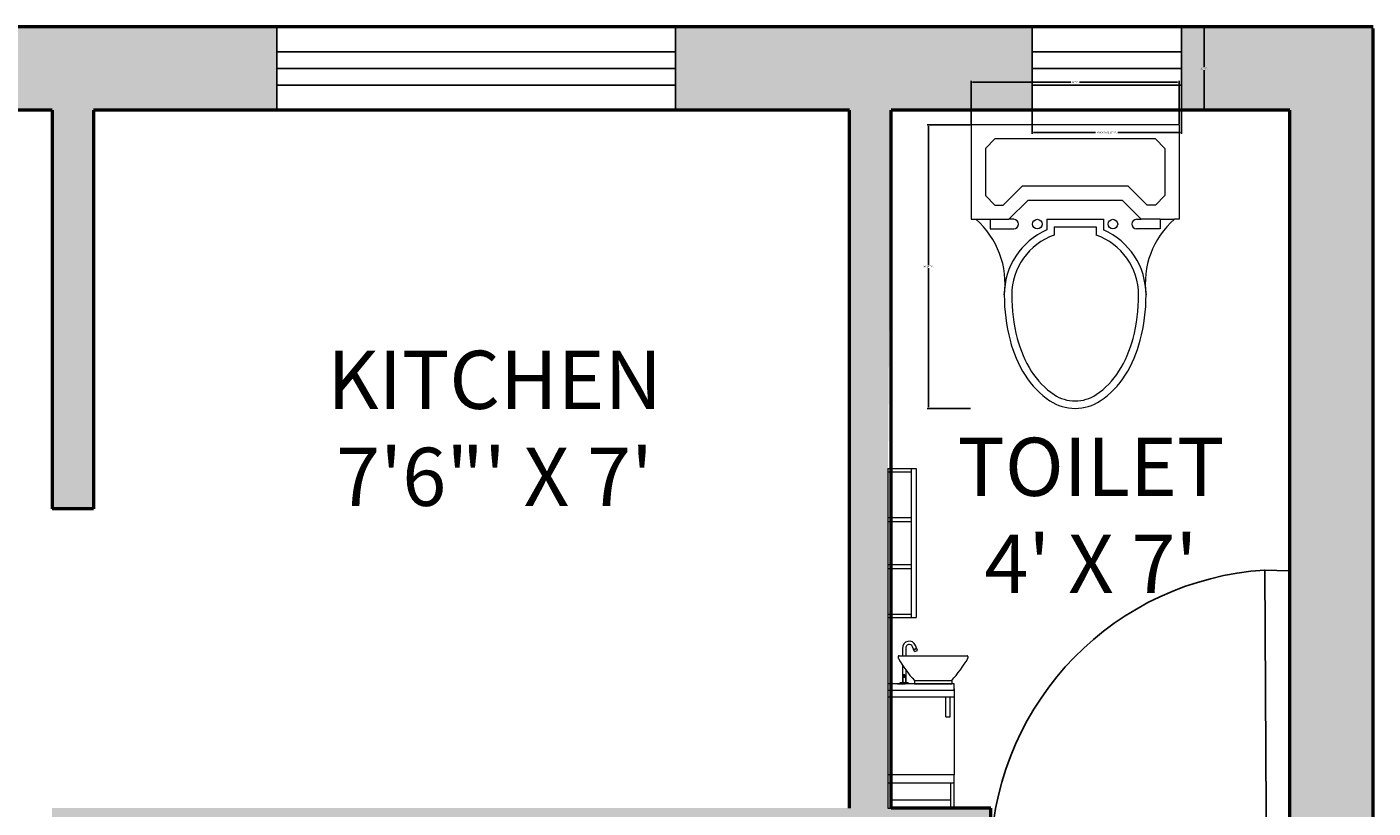
# Model space of a CAD drawing. Units: inches. Extents: x 1771 to 3025, y 319 to 889.
# Tile 12 of 35: x 1939 to 2101, y 795 to 889. Entities that reach past the tile are written whole.
import ezdxf

# ---------------------------------------------------------------- set-up
doc = ezdxf.new("R2010")
doc.units = ezdxf.units.IN
doc.header["$MEASUREMENT"] = 0
for name, color, linetype, lineweight in [('A-ANNO-DIMS', 2, 'Continuous', 18), ('A-AREA-IDEN', 241, 'Continuous', 25), ('A-DOOR', 4, 'Continuous', 25), ('A-FLOR-FIXT', 8, 'Continuous', 18), ('A-GLAZ', 40, 'Continuous', 25), ('A-WALL', 7, 'Continuous', 50), ('A-WALL-PATT', 254, 'Continuous', 13)]:
    doc.layers.add(name, color=color, linetype=linetype, lineweight=lineweight)
doc.styles.get("Standard").update_dxf_attribs({"font": 'arial.ttf'})
doc.dimstyles.get("Standard").update_dxf_attribs({"dimtxt": 0.18, "dimasz": 0.18, "dimexe": 0.18, "dimexo": 0.0625, "dimgap": 0.09, "dimtad": 0, "dimtih": 1, "dimtoh": 1, "dimdec": 4, "dimzin": 0, "dimdsep": 46, "dimtxsty": 'Standard', "dimcen": 0.09, "dimadec": 0, "dimazin": 0, "dimtfac": 1, "dimtdec": 4, "dimtofl": 0, "dimtmove": 0, "dimatfit": 3, "dimfxl": 1, "dimtolj": 1, "dimtzin": 0, "dimarcsym": 0})

# ---------------------------------------------------------------- blocks, each defined once
blk = doc.blocks.new('A$C098B081F')
for p, q in [((558.8, 762), (0, 762)), ((0, 762), (0, 508)), ((558.8, 762), (558.8, 508)), ((63.5, 723.9), (38.1, 698.5)), ((495.3, 723.9), (63.5, 723.9)), ((520.7, 698.5), (495.3, 723.9)), ((38.1, 698.5), (38.1, 571.5)), ((520.7, 698.5), (520.7, 571.5)), ((136.6, 596.9), (85.8, 546.1)), ((422.2, 596.9), (136.6, 596.9)), ((422.2, 596.9), (473, 546.1)), ((38.1, 571.5), (63.5, 546.1)), ((63.5, 546.1), (85.8, 546.1)), ((152.4, 558.8), (101.6, 508)), ((406.4, 558.8), (152.4, 558.8)), ((406.4, 558.8), (457.2, 508)), ((495.3, 546.1), (473, 546.1)), ((495.3, 546.1), (520.7, 571.5)), ((0, 508), (12.7, 508)), ((12.7, 508), (101.6, 508)), ((50.8, 508), (50.8, 482.6)), ((50.8, 508), (101.6, 508)), ((114.3, 508), (101.6, 508)), ((203.2, 508), (203.2, 479.4)), ((203.2, 508), (355.6, 508)), ((355.6, 508), (355.6, 479.4)), ((444.5, 508), (457.2, 508)), ((508, 508), (457.2, 508)), ((508, 508), (546.1, 508)), ((508, 508), (508, 482.6)), ((558.8, 508), (546.1, 508)), ((50.8, 482.6), (114.3, 482.6)), ((223.2, 488), (223.2, 465.8)), ((223.2, 488), (335.6, 488)), ((335.6, 488), (335.6, 465.8)), ((508, 482.6), (444.5, 482.6))]:
    blk.add_line(p, q)
for centre in [(177.8, 495.3), (381, 495.3)]:
    blk.add_circle(centre, 12.7)
for centre, radius, start, end in [((-137.5, 335.8), 228.5, 352.2011, 48.911), ((114.3, 495.3), 12.7, 270, 90), ((444.5, 495.3), 12.7, 90, 270), ((696.3, 335.8), 228.5, 131.089, 187.7989), ((279.4, 304.8), 190.5, 113.5782, 180), ((279.4, 304.8), 190.5, 0, 66.4218), ((279.4, 304.8), 170.5, 109.2456, 180), ((279.4, 304.8), 170.5, 0, 70.7544), ((574.9, 304.8), 486, 180, 194.5143), ((574.9, 304.8), 466, 180, 194.5143), ((-16.1, 304.8), 466, 345.4857, 360), ((-16.1, 304.8), 486, 345.4857, 360), ((429.2, 267.1), 335.5, 194.5143, 212.0054), ((429.2, 267.1), 315.5, 194.5143, 212.0054), ((129.6, 267.1), 315.5, 327.9946, 345.4857), ((129.6, 267.1), 335.5, 327.9946, 345.4857), ((337.2, 209.6), 227, 212.0054, 236.4659), ((337.2, 209.6), 207, 212.0054, 236.4659), ((221.6, 209.6), 207, 303.5341, 327.9946), ((221.6, 209.6), 227, 303.5341, 327.9946), ((279.4, 122.4), 102.4, 236.4659, 270), ((279.4, 122.4), 102.4, 270, 303.5341), ((279.4, 122.4), 122.4, 236.4659, 270), ((279.4, 122.4), 122.4, 270, 303.5341)]:
    blk.add_arc(centre, radius, start, end)
blk = doc.blocks.new('A$C3EAC730C')
for p, q in [((0, 2.05), (0.17, 2.05)), ((0, 2.05), (0, 0.2)), ((0.14, 2.05), (0.14, 1.15)), ((0.17, 2.05), (0.17, 1.15)), ((0, 2.03), (0.14, 2.03)), ((0, 1.7542), (0.14, 1.7542)), ((0, 1.7292), (0.14, 1.7292)), ((0, 1.4708), (0.14, 1.4708)), ((0, 1.4458), (0.14, 1.4458)), ((0, 1.17), (0.14, 1.17)), ((0, 1.15), (0.17, 1.15)), ((0.1787, 0.9521), (0.1666, 0.9819)), ((0.0627, 0.915), (0.0627, 0.9063)), ((0.0677, 0.92), (0.4777, 0.92)), ((0.0877, 0.964), (0.0877, 0.92)), ((0.1077, 0.9647), (0.1077, 0.92)), ((0.1601, 0.9446), (0.1481, 0.9744)), ((0.1545, 0.9582), (0.1731, 0.9657)), ((0.1552, 0.9563), (0.1739, 0.9639)), ((0.1601, 0.9446), (0.1787, 0.9521)), ((0.4827, 0.915), (0.4827, 0.9063)), ((0.4827, 0.915), (0.4827, 0.9063)), ((0.0877, 0.8637), (0.0877, 0.756)), ((0.1077, 0.8346), (0.1077, 0.756)), ((0.4, 0.75), (0, 0.75)), ((0.0577, 0.75), (0.1037, 0.75)), ((0.0727, 0.756), (0.0727, 0.75)), ((0.1227, 0.756), (0.0727, 0.756)), ((0.0902, 0.7905), (0.1052, 0.7905)), ((0.0902, 0.7905), (0.0902, 0.756)), ((0.0947, 0.8022), (0.0947, 0.7905)), ((0.1007, 0.8022), (0.1007, 0.7905)), ((0.1052, 0.7905), (0.1052, 0.756)), ((0.1227, 0.756), (0.1227, 0.75)), ((0.1602, 0.77), (0.1602, 0.75)), ((0.1602, 0.77), (0.3852, 0.77)), ((0.1602, 0.75), (0.3852, 0.75)), ((0.3852, 0.77), (0.3852, 0.75)), ((0.4, 0.71), (0.4, 0.75)), ((0.4, 0.71), (0, 0.71)), ((0.4, 0.67), (0, 0.67)), ((0.35, 0.55), (0.35, 0.67)), ((0.375, 0.55), (0.375, 0.67)), ((0.4, 0.72), (0.4, 0.2)), ((0.35, 0.55), (0.375, 0.55)), ((0.4, 0.2), (0, 0.2)), ((0, 0.2), (0, 0)), ((0.4, 0), (0.4, 0.2)), ((0.4, 0.15), (0, 0.15)), ((0.02, 0.15), (0.02, 0)), ((0.38, 0), (0.38, 0.15)), ((0, 0), (0.4, 0)), ((0.02, 0.05), (0.38, 0.05))]:
    blk.add_line(p, q)
blk.add_circle((0.0977, 0.804), 0.0035)
for centre, radius, start, end in [((0.1286, 0.9665), 0.041, 22.01327, 183.41193), ((0.1286, 0.9665), 0.021, 22.01327, 184.76808), ((0.0677, 0.915), 0.005, 90, 180), ((0.0677, 0.9063), 0.005, 180, 209.45502), ((0.7052, 1.2664), 0.7372, 209.45502, 222.32259), ((-0.1599, 1.2664), 0.7372, 317.67741, 330.54498), ((0.4777, 0.915), 0.005, 0, 90), ((0.4777, 0.9063), 0.005, 330.54498, 0)]:
    blk.add_arc(centre, radius, start, end)
blk = doc.blocks.new('DOOR-35')
blk.add_lwpolyline([(35.88, 36.19), (32.96, 36.3), (33.16, 0), (36, 0.05)], close=True)
blk.add_arc((35.23, 1.11), 35.26, 93.6879, 177.4925)
blk = doc.blocks.new('WIN-48')
for p, q in [((0, 0), (0, 10)), ((48, 0), (48, 10)), ((0, 7), (48, 7)), ((0, 5), (48, 5)), ((0, 3), (48, 3))]:
    blk.add_line(p, q)
blk = doc.blocks.new('WIN-18')
for p, q in [((0, 0), (0, 10)), ((18, 0), (18, 10)), ((0, 7), (18, 7)), ((0, 5), (18, 5)), ((0, 3), (18, 3))]:
    blk.add_line(p, q)
blk = doc.blocks.new('*D26')
at = {"layer": 'A-ANNO-DIMS', "color": 0, "lineweight": -2, "transparency": 16777216}
for p, q in [((2059.68, 878.57), (2059.68, 875.75)), ((2077.68, 878.57), (2077.68, 875.75)), ((2059.86, 875.93), (2067.33, 875.93)), ((2077.5, 875.93), (2070.02, 875.93))]:
    blk.add_line(p, q, dxfattribs=at)
at = {"layer": 'A-ANNO-DIMS', "color": 0, "transparency": 16777216}
for points in [[(2059.86, 875.96), (2059.86, 875.9), (2059.68, 875.93)], [(2077.5, 875.96), (2077.5, 875.9), (2077.68, 875.93)]]:
    blk.add_solid(points, dxfattribs=at)
at = {"layer": 'Defpoints', "color": 0, "transparency": 16777216}
for p in [(2059.68, 878.63), (2077.68, 878.63), (2077.68, 875.93)]:
    blk.add_point(p, dxfattribs=at)
at = {"layer": 'A-ANNO-DIMS', "color": 0, "transparency": 16777216, "insert": (2068.68, 875.93), "char_height": 0.18, "attachment_point": 5}
blk.add_mtext('\\A1;WINDOW W2 18 TYP.', dxfattribs=at)
blk = doc.blocks.new('*D27')
at = {"layer": 'A-ANNO-DIMS', "color": 0, "lineweight": -2, "transparency": 16777216}
for p, q in [((2077.74, 888.63), (2080.56, 888.63)), ((2080.38, 888.45), (2080.38, 883.82)), ((2080.38, 878.81), (2080.38, 883.45)), ((2077.74, 878.63), (2080.56, 878.63))]:
    blk.add_line(p, q, dxfattribs=at)
at = {"layer": 'A-ANNO-DIMS', "color": 0, "transparency": 16777216}
for points in [[(2080.35, 888.45), (2080.41, 888.45), (2080.38, 888.63)], [(2080.35, 878.81), (2080.41, 878.81), (2080.38, 878.63)]]:
    blk.add_solid(points, dxfattribs=at)
at = {"layer": 'Defpoints', "color": 0, "transparency": 16777216}
for p in [(2077.68, 888.63), (2080.38, 888.63), (2077.68, 878.63)]:
    blk.add_point(p, dxfattribs=at)
at = {"layer": 'A-ANNO-DIMS', "color": 0, "transparency": 16777216, "insert": (2080.38, 883.63), "char_height": 0.18, "attachment_point": 5}
blk.add_mtext('\\A1;10 TYP.', dxfattribs=at)
blk = doc.blocks.new('*D56')
at = {"layer": 'A-ANNO-DIMS', "color": 0, "lineweight": -2, "transparency": 16777216}
for p, q in [((2052.28, 876.86), (2047.05, 876.86)), ((2047.23, 876.68), (2047.23, 859.98)), ((2047.23, 842.91), (2047.23, 859.61)), ((2052.28, 842.73), (2047.05, 842.73))]:
    blk.add_line(p, q, dxfattribs=at)
at = {"layer": 'A-ANNO-DIMS', "color": 0, "transparency": 16777216}
for points in [[(2047.2, 876.68), (2047.26, 876.68), (2047.23, 876.86)], [(2047.2, 842.91), (2047.26, 842.91), (2047.23, 842.73)]]:
    blk.add_solid(points, dxfattribs=at)
at = {"layer": 'Defpoints', "color": 0, "transparency": 16777216}
for p in [(2047.23, 876.86), (2052.35, 876.86), (2052.35, 842.73)]:
    blk.add_point(p, dxfattribs=at)
at = {"layer": 'A-ANNO-DIMS', "color": 0, "transparency": 16777216, "insert": (2047.23, 859.8), "char_height": 0.18, "attachment_point": 5}
blk.add_mtext('\\A1;WC 34 TYP.', dxfattribs=at)
blk = doc.blocks.new('*D57')
at = {"layer": 'A-ANNO-DIMS', "color": 0, "lineweight": -2, "transparency": 16777216}
for p, q in [((2052.35, 876.93), (2052.35, 882.16)), ((2052.53, 881.98), (2064.33, 881.98)), ((2077.2, 881.98), (2065.39, 881.98)), ((2077.38, 876.93), (2077.38, 882.16))]:
    blk.add_line(p, q, dxfattribs=at)
at = {"layer": 'A-ANNO-DIMS', "color": 0, "transparency": 16777216}
for points in [[(2052.53, 882.01), (2052.53, 881.95), (2052.35, 881.98)], [(2077.2, 882.01), (2077.2, 881.95), (2077.38, 881.98)]]:
    blk.add_solid(points, dxfattribs=at)
at = {"layer": 'Defpoints', "color": 0, "transparency": 16777216}
for p in [(2077.38, 881.98), (2052.35, 876.86), (2077.38, 876.86)]:
    blk.add_point(p, dxfattribs=at)
at = {"layer": 'A-ANNO-DIMS', "color": 0, "transparency": 16777216, "insert": (2064.86, 881.98), "char_height": 0.18, "attachment_point": 5}
blk.add_mtext('\\A1;25 TYP.', dxfattribs=at)

msp = doc.modelspace()

# ---------------------------------------------------------------- hatches: boundary and pattern name
at = {"layer": 'A-WALL-PATT'}
h = msp.add_hatch(color=256, dxfattribs=at)
h.dxf.hatch_style = 1
h.paths.add_polyline_path([(1870.72, 888.63), (1799.72, 888.63), (1799.72, 878.63), (1870.72, 878.63)])
h.paths.add_polyline_path([(1968.77, 888.63), (1918.72, 888.63), (1918.72, 878.63), (1941.72, 878.63), (1941.72, 830.63), (1946.72, 830.63), (1946.72, 878.63), (1968.77, 878.63)])
h.paths.add_polyline_path([(2059.68, 888.63), (2016.77, 888.63), (2016.77, 878.63), (2037.72, 878.63), (2037.72, 794.63), (1941.72, 794.63), (1941.72, 758.63), (1941.72, 664.63), (1946.72, 664.63), (1946.72, 712), (1946.72, 789.63), (2054.72, 789.63), (2054.72, 794.63), (2042.33, 794.63), (2042.33, 798.62), (2042.33, 835.5), (2042.72, 878.63), (2059.68, 878.63)])
h.paths.add_polyline_path([(2100.72, 888.63), (2077.68, 888.63), (2077.68, 878.63), (2090.72, 878.63), (2090.72, 789.63), (2090.72, 768.61), (2100.72, 768.61)])
h.paths.add_polyline_path([(2100.72, 720.61), (2090.72, 720.61), (2090.72, 669.63), (1982.72, 669.63), (1982.72, 664.63), (2001.72, 664.63), (2001.72, 652.63), (2006.72, 652.63), (2006.72, 664.63), (2049.52, 664.63, -0.385549), (2050.52, 664.63), (2090.72, 664.63), (2090.72, 649.17), (2100.72, 649.17)])
edge = h.paths.add_edge_path()
edge.add_line((2100.72, 631.17), (2090.72, 631.17))
edge.add_line((2090.72, 631.17), (2090.72, 616.63))
edge.add_line((2090.72, 616.63), (2001.72, 616.63))
edge.add_line((2001.72, 616.63), (1982.72, 616.63))
edge.add_line((1982.72, 616.63), (1982.72, 611.63))
edge.add_line((1982.72, 611.63), (2024.67, 611.63))
edge.add_spline(control_points=[(2024.67, 611.63), (2027.58, 612.87), (2030.01, 613.31), (2032.47, 613.72)], knot_values=[484.321569, 484.321569, 484.321569, 484.321569, 625.498764, 625.498764, 625.498764, 625.498764], degree=3, periodic=0)
edge.add_line((2032.47, 613.72), (2033.2, 613.72))
edge.add_spline(control_points=[(2033.2, 613.72), (2035.66, 613.31), (2039.46, 612.87), (2042.2, 611.63)], knot_values=[484.321569, 484.321569, 484.321569, 484.321569, 625.498764, 625.498764, 625.498764, 625.498764], degree=3, periodic=0)
edge.add_line((2042.2, 611.63), (2090.72, 611.63))
edge.add_line((2090.72, 611.63), (2090.72, 581.11))
edge.add_line((2090.72, 581.11), (2100.72, 581.11))
edge.add_line((2100.72, 581.11), (2100.72, 631.17))
h.paths.add_polyline_path([(2100.72, 533.11), (2090.72, 533.11), (2090.72, 479.63), (1946.72, 479.63), (1946.72, 616.63), (1936.72, 616.63), (1936.72, 543.63), (1845.72, 543.63), (1845.72, 533.63), (1936.72, 533.63), (1936.72, 469.63), (2090.72, 469.63), (2090.72, 452.76), (2100.72, 452.76)])
h.paths.add_polyline_path([(2100.72, 404.76), (2090.72, 404.76), (2090.72, 393.63), (1936.72, 393.63), (1936.72, 383.63), (2100.72, 383.63)])
h.paths.add_polyline_path([(1905.72, 758.63), (1835.47, 758.63), (1835.47, 758.63), (1813.44, 758.63), (1809.72, 758.63), (1809.72, 842.59, -0.008336), (1808.42, 842.63), (1799.72, 842.63), (1799.72, 690.58), (1809.72, 690.58), (1809.72, 753.63), (1905.72, 753.63)])
h.paths.add_polyline_path([(1809.72, 642.58), (1799.72, 642.58), (1799.72, 533.63), (1809.72, 533.63), (1809.72, 581)])

# ---------------------------------------------------------------- linework, layer by layer
at = {"layer": 'A-WALL'}
for p, q in [((2100.72, 888.63), (1799.72, 888.63)), ((2100.72, 383.63), (2100.72, 888.43)), ((1941.72, 878.63), (1799.72, 878.63)), ((1941.72, 878.63), (1941.72, 830.63)), ((1946.72, 878.63), (1946.72, 830.63)), ((2037.72, 878.63), (1946.72, 878.63)), ((2037.72, 794.63), (2037.72, 878.63)), ((2090.72, 878.63), (2042.72, 878.63)), ((2042.72, 794.63), (2042.72, 878.63)), ((2090.72, 789.63), (2090.72, 878.63)), ((1946.72, 830.63), (1941.72, 830.63)), ((2054.72, 794.63), (2042.72, 794.63)), ((2054.72, 789.63), (2054.72, 794.63))]:
    msp.add_line(p, q, dxfattribs=at)

# ---------------------------------------------------------------- block references
at = {"layer": 'A-DOOR'}
msp.add_blockref('DOOR-35', (2054.72, 786.98), dxfattribs=at)
at = {"layer": 'A-FLOR-FIXT'}
for name, p, xscale, yscale, zscale in [('A$C098B081F', (2052.35, 842.73), 0.0447923195545138, 0.0447923195545138, 0.0447923195545138), ('A$C3EAC730C', (2042.33, 794.63), 19.93356852258053, 19.93356852258053, 19.93356852258053)]:
    msp.add_blockref(name, p, dxfattribs=dict(at, xscale=xscale, yscale=yscale, zscale=zscale))
at = {"layer": 'A-GLAZ'}
for name, p in [('WIN-48', (1968.77, 878.63)), ('WIN-18', (2059.68, 878.63))]:
    msp.add_blockref(name, p, dxfattribs=at)

# ---------------------------------------------------------------- texts
at = {"layer": 'A-AREA-IDEN', "char_height": 7, "attachment_point": 1}
for s, insert in [('\\pxqc;KITCHEN\\P7\'6"\' X 7\'', (1952.26, 849.67)), ("\\pxqc;TOILET\\P4' X 7'", (2024.03, 839.2))]:
    msp.add_mtext_dynamic_manual_height_columns(s, width=85.4611, gutter_width=1, heights=[0], dxfattribs=dict(at, insert=insert))

# ---------------------------------------------------------------- dimensions: what is measured, and where the dimension line sits
at = {"layer": 'A-ANNO-DIMS'}
for base, p1, p2, text, picture, middle in [((2080.38, 888.63), (2077.68, 878.63), (2077.68, 888.63), '<> TYP.', '*D27', (2080.38, 883.63)), ((2047.23, 876.86), (2052.35, 842.73), (2052.35, 876.86), 'WC <> TYP.', '*D56', (2047.23, 859.8))]:
    dim = msp.add_linear_dim(base=base, p1=p1, p2=p2, angle=90, text=text, dimstyle='Standard', override={"dimdec": 0, "dimrnd": 0, "dimzin": 0, "dimlunit": 2}, dxfattribs=at)
    dim.commit()
    dim.dimension.update_dxf_attribs({"geometry": picture, "text_midpoint": middle})
for base, p1, p2, text, picture, middle in [((2077.38, 881.98), (2052.35, 876.86), (2077.38, 876.86), '<> TYP.', '*D57', (2064.86, 881.98)), ((2077.68, 875.93), (2059.68, 878.63), (2077.68, 878.63), 'WINDOW W2 <> TYP.', '*D26', (2068.68, 875.93))]:
    dim = msp.add_linear_dim(base=base, p1=p1, p2=p2, text=text, dimstyle='Standard', override={"dimdec": 0, "dimrnd": 0, "dimzin": 0, "dimlunit": 2}, dxfattribs=at)
    dim.commit()
    dim.dimension.update_dxf_attribs({"geometry": picture, "text_midpoint": middle})

doc.saveas('drawing.dxf')
